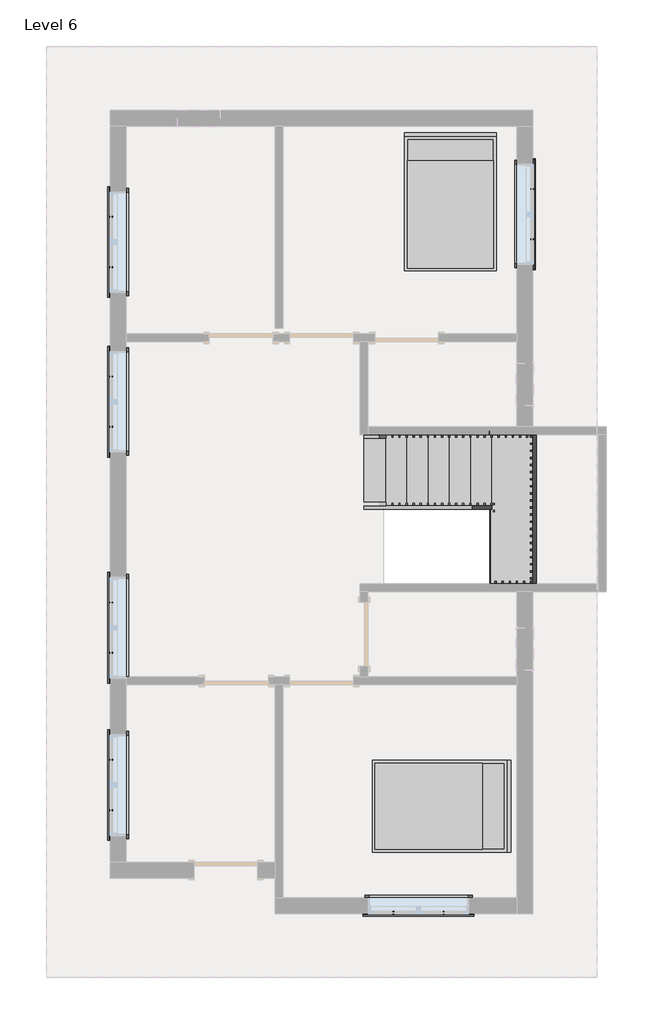
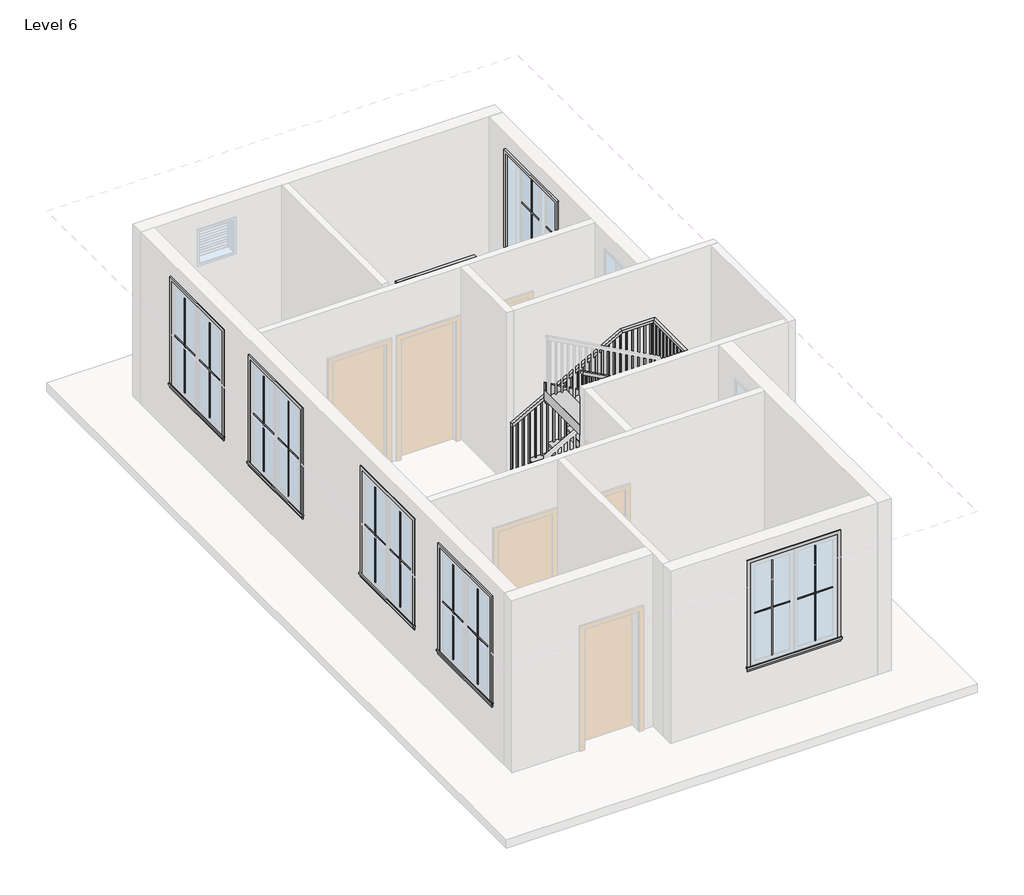
# One storey, part 2 of 2: 24 proxies, 5 members, 2 furniture elements, 1 railing, 1 stair flight.
"""IFC4 building model written with IfcOpenShell, lengths in millimetres."""

from ifc_helpers import new_model, si_unit, frame, origin, place, context, project, spatial, polyline, outline, extrude, faceted_brep, transform, mapped, element, save
from components import muntin_pattern_2x2_muntin_pattern_2x2_bff912c5, muntin_pattern_2x2_muntin_pattern_2x2_c2194282, trim_window_exterior_flat_with_sill_e04b3088, trim_window_interior_flat_picture_frame_2a7685fe, bed_17739_bed_17739_15c61121, stair_flight_57dbdc02

model = new_model("IFC4")

# Units and contexts
model_context = context("Model", 3, world=origin())
ifc_project = project(units=[si_unit("LENGTHUNIT", "METRE", prefix="MILLI")], contexts=[model_context])

# Site, building, storey
site = spatial("IfcSite", under=ifc_project)
building = spatial("IfcBuilding", under=site)
storey = spatial("IfcBuildingStorey", under=building, Name="Level 6", Elevation=12801.6)

# Proxies
placement = place(None, origin())
muntin_pattern_2x2_muntin_pattern_2x2_shape = muntin_pattern_2x2_muntin_pattern_2x2_bff912c5(model_context)
element("IfcBuildingElementProxy", 1, Name="Muntin Pattern_2x2 : Muntin Pattern_2x2", ObjectType="Muntin Pattern_2x2 : Muntin Pattern_2x2", at=placement, inside=storey, context=model_context, shape_type="MappedRepresentation", body=[
    mapped(muntin_pattern_2x2_muntin_pattern_2x2_shape, transform((-4796.6888307, -4528.6107799, 13785.85), x_axis=(0.0, 1.0, 0.0), y_axis=(-1.0, 0.0, 0.0), z_axis=(0.0, 0.0, 1.0))),
])
element("IfcBuildingElementProxy", 2, Name="Muntin Pattern_2x2 : Muntin Pattern_2x2", ObjectType="Muntin Pattern_2x2 : Muntin Pattern_2x2", at=placement, inside=storey, context=model_context, shape_type="MappedRepresentation", body=[
    mapped(muntin_pattern_2x2_muntin_pattern_2x2_shape, transform((-4796.6888307, -2274.3607799, 13785.85), x_axis=(0.0, 1.0, 0.0), y_axis=(-1.0, 0.0, 0.0), z_axis=(0.0, 0.0, 1.0))),
])
element("IfcBuildingElementProxy", 3, Name="Muntin Pattern_2x2 : Muntin Pattern_2x2", ObjectType="Muntin Pattern_2x2 : Muntin Pattern_2x2", at=placement, inside=storey, context=model_context, shape_type="MappedRepresentation", body=[
    mapped(muntin_pattern_2x2_muntin_pattern_2x2_shape, transform((-26.2513307, -6000.2232799, 13785.85), x_axis=(-1.0, 0.0, 0.0), y_axis=(0.0, -1.0, 0.0), z_axis=(0.0, 0.0, 1.0))),
])
element("IfcBuildingElementProxy", 4, Name="Muntin Pattern_2x2 : Muntin Pattern_2x2", ObjectType="Muntin Pattern_2x2 : Muntin Pattern_2x2", at=placement, inside=storey, context=model_context, shape_type="MappedRepresentation", body=[
    mapped(muntin_pattern_2x2_muntin_pattern_2x2_shape, transform((1242.1611693, 4370.9142201, 13785.85), x_axis=(0.0, -1.0, 0.0), y_axis=(1.0, 0.0, 0.0), z_axis=(0.0, 0.0, 1.0))),
])
element("IfcBuildingElementProxy", 5, Name="Muntin Pattern_2x2 : Muntin Pattern_2x2", ObjectType="Muntin Pattern_2x2 : Muntin Pattern_2x2", at=placement, inside=storey, context=model_context, shape_type="MappedRepresentation", body=[
    mapped(muntin_pattern_2x2_muntin_pattern_2x2_shape, transform((-4796.6888307, 3250.1392201, 13785.85), x_axis=(0.0, 1.0, 0.0), y_axis=(-1.0, 0.0, 0.0), z_axis=(0.0, 0.0, 1.0))),
])
element("IfcBuildingElementProxy", 6, Name="Muntin Pattern_2x2 : Muntin Pattern_2x2", ObjectType="Muntin Pattern_2x2 : Muntin Pattern_2x2", at=placement, inside=storey, context=model_context, shape_type="MappedRepresentation", body=[
    mapped(muntin_pattern_2x2_muntin_pattern_2x2_shape, transform((-4796.6888307, 964.1392201, 13785.85), x_axis=(0.0, 1.0, 0.0), y_axis=(-1.0, 0.0, 0.0), z_axis=(0.0, 0.0, 1.0))),
])
muntin_pattern_2x2_muntin_pattern_2x2_2_shape = muntin_pattern_2x2_muntin_pattern_2x2_c2194282(model_context)
element("IfcBuildingElementProxy", 7, Name="Muntin Pattern_2x2 : Muntin Pattern_2x2", ObjectType="Muntin Pattern_2x2 : Muntin Pattern_2x2", at=placement, inside=storey, context=model_context, shape_type="MappedRepresentation", body=[
    mapped(muntin_pattern_2x2_muntin_pattern_2x2_2_shape, transform((-4796.6888307, -3807.8857799, 13785.85), x_axis=(0.0, -1.0, 0.0), y_axis=(1.0, 0.0, 0.0), z_axis=(0.0, 0.0, 1.0))),
])
element("IfcBuildingElementProxy", 8, Name="Muntin Pattern_2x2 : Muntin Pattern_2x2", ObjectType="Muntin Pattern_2x2 : Muntin Pattern_2x2", at=placement, inside=storey, context=model_context, shape_type="MappedRepresentation", body=[
    mapped(muntin_pattern_2x2_muntin_pattern_2x2_2_shape, transform((-4796.6888307, -1553.6357799, 13785.85), x_axis=(0.0, -1.0, 0.0), y_axis=(1.0, 0.0, 0.0), z_axis=(0.0, 0.0, 1.0))),
])
element("IfcBuildingElementProxy", 9, Name="Muntin Pattern_2x2 : Muntin Pattern_2x2", ObjectType="Muntin Pattern_2x2 : Muntin Pattern_2x2", at=placement, inside=storey, context=model_context, shape_type="MappedRepresentation", body=[
    mapped(muntin_pattern_2x2_muntin_pattern_2x2_2_shape, transform((-746.9763307, -6000.2232799, 13785.85), x_axis=(1.0, 0.0, 0.0), y_axis=(0.0, 1.0, 0.0), z_axis=(0.0, 0.0, 1.0))),
])
element("IfcBuildingElementProxy", 10, Name="Muntin Pattern_2x2 : Muntin Pattern_2x2", ObjectType="Muntin Pattern_2x2 : Muntin Pattern_2x2", at=placement, inside=storey, context=model_context, shape_type="MappedRepresentation", body=[
    mapped(muntin_pattern_2x2_muntin_pattern_2x2_2_shape, transform((1242.1611693, 3650.1892201, 13785.85), x_axis=(0.0, 1.0, 0.0), y_axis=(-1.0, 0.0, 0.0), z_axis=(0.0, 0.0, 1.0))),
])
element("IfcBuildingElementProxy", 11, Name="Muntin Pattern_2x2 : Muntin Pattern_2x2", ObjectType="Muntin Pattern_2x2 : Muntin Pattern_2x2", at=placement, inside=storey, context=model_context, shape_type="MappedRepresentation", body=[
    mapped(muntin_pattern_2x2_muntin_pattern_2x2_2_shape, transform((-4796.6888307, 3970.8642201, 13785.85), x_axis=(0.0, -1.0, 0.0), y_axis=(1.0, 0.0, 0.0), z_axis=(0.0, 0.0, 1.0))),
])
element("IfcBuildingElementProxy", 12, Name="Muntin Pattern_2x2 : Muntin Pattern_2x2", ObjectType="Muntin Pattern_2x2 : Muntin Pattern_2x2", at=placement, inside=storey, context=model_context, shape_type="MappedRepresentation", body=[
    mapped(muntin_pattern_2x2_muntin_pattern_2x2_2_shape, transform((-4796.6888307, 1684.8642201, 13785.85), x_axis=(0.0, -1.0, 0.0), y_axis=(1.0, 0.0, 0.0), z_axis=(0.0, 0.0, 1.0))),
])
trim_window_exterior_flat_with_sill_shape = trim_window_exterior_flat_with_sill_e04b3088(model_context)
element("IfcBuildingElementProxy", 13, Name="Trim-Window-Exterior-Flat : with Sill", ObjectType="Trim-Window-Exterior-Flat : with Sill", at=placement, inside=storey, context=model_context, shape_type="MappedRepresentation", body=[
    mapped(trim_window_exterior_flat_with_sill_shape, transform((-4806.2138307, -4168.2482799, 15544.8), x_axis=(0.0, -1.0, 0.0), y_axis=(0.0, 0.0, 1.0), z_axis=(-1.0, 0.0, 0.0))),
])
element("IfcBuildingElementProxy", 14, Name="Trim-Window-Exterior-Flat : with Sill", ObjectType="Trim-Window-Exterior-Flat : with Sill", at=placement, inside=storey, context=model_context, shape_type="MappedRepresentation", body=[
    mapped(trim_window_exterior_flat_with_sill_shape, transform((-4806.2138307, -1913.9982799, 15544.8), x_axis=(0.0, -1.0, 0.0), y_axis=(0.0, 0.0, 1.0), z_axis=(-1.0, 0.0, 0.0))),
])
element("IfcBuildingElementProxy", 15, Name="Trim-Window-Exterior-Flat : with Sill", ObjectType="Trim-Window-Exterior-Flat : with Sill", at=placement, inside=storey, context=model_context, shape_type="MappedRepresentation", body=[
    mapped(trim_window_exterior_flat_with_sill_shape, transform((-386.6138307, -6009.7482799, 15544.8), x_axis=(1.0, 0.0, 0.0), y_axis=(0.0, 0.0, 1.0), z_axis=(0.0, -1.0, 0.0))),
])
element("IfcBuildingElementProxy", 16, Name="Trim-Window-Exterior-Flat : with Sill", ObjectType="Trim-Window-Exterior-Flat : with Sill", at=placement, inside=storey, context=model_context, shape_type="MappedRepresentation", body=[
    mapped(trim_window_exterior_flat_with_sill_shape, transform((1251.6861693, 4010.5517201, 15544.8), x_axis=(0.0, 1.0, 0.0), y_axis=(0.0, 0.0, 1.0), z_axis=(1.0, 0.0, 0.0))),
])
element("IfcBuildingElementProxy", 17, Name="Trim-Window-Exterior-Flat : with Sill", ObjectType="Trim-Window-Exterior-Flat : with Sill", at=placement, inside=storey, context=model_context, shape_type="MappedRepresentation", body=[
    mapped(trim_window_exterior_flat_with_sill_shape, transform((-4806.2138307, 3610.5017201, 15544.8), x_axis=(0.0, -1.0, 0.0), y_axis=(0.0, 0.0, 1.0), z_axis=(-1.0, 0.0, 0.0))),
])
element("IfcBuildingElementProxy", 18, Name="Trim-Window-Exterior-Flat : with Sill", ObjectType="Trim-Window-Exterior-Flat : with Sill", at=placement, inside=storey, context=model_context, shape_type="MappedRepresentation", body=[
    mapped(trim_window_exterior_flat_with_sill_shape, transform((-4806.2138307, 1324.5017201, 15544.8), x_axis=(0.0, -1.0, 0.0), y_axis=(0.0, 0.0, 1.0), z_axis=(-1.0, 0.0, 0.0))),
])
trim_window_interior_flat_picture_frame_shape = trim_window_interior_flat_picture_frame_2a7685fe(model_context)
element("IfcBuildingElementProxy", 19, Name="Trim-Window-Interior-Flat : Picture Frame", ObjectType="Trim-Window-Interior-Flat : Picture Frame", at=placement, inside=storey, context=model_context, shape_type="MappedRepresentation", body=[
    mapped(trim_window_interior_flat_picture_frame_shape, transform((-4577.6138307, -4168.2482799, 15544.8), x_axis=(0.0, 1.0, 0.0), y_axis=(0.0, 0.0, 1.0), z_axis=(1.0, 0.0, 0.0))),
])
element("IfcBuildingElementProxy", 20, Name="Trim-Window-Interior-Flat : Picture Frame", ObjectType="Trim-Window-Interior-Flat : Picture Frame", at=placement, inside=storey, context=model_context, shape_type="MappedRepresentation", body=[
    mapped(trim_window_interior_flat_picture_frame_shape, transform((-4577.6138307, -1913.9982799, 15544.8), x_axis=(0.0, 1.0, 0.0), y_axis=(0.0, 0.0, 1.0), z_axis=(1.0, 0.0, 0.0))),
])
element("IfcBuildingElementProxy", 21, Name="Trim-Window-Interior-Flat : Picture Frame", ObjectType="Trim-Window-Interior-Flat : Picture Frame", at=placement, inside=storey, context=model_context, shape_type="MappedRepresentation", body=[
    mapped(trim_window_interior_flat_picture_frame_shape, transform((-386.6138307, -5781.1482799, 15544.8), x_axis=(-1.0, 0.0, 0.0), y_axis=(0.0, 0.0, 1.0), z_axis=(0.0, 1.0, 0.0))),
])
element("IfcBuildingElementProxy", 22, Name="Trim-Window-Interior-Flat : Picture Frame", ObjectType="Trim-Window-Interior-Flat : Picture Frame", at=placement, inside=storey, context=model_context, shape_type="MappedRepresentation", body=[
    mapped(trim_window_interior_flat_picture_frame_shape, transform((1023.0861693, 4010.5517201, 15544.8), x_axis=(0.0, -1.0, 0.0), y_axis=(0.0, 0.0, 1.0), z_axis=(-1.0, 0.0, 0.0))),
])
element("IfcBuildingElementProxy", 23, Name="Trim-Window-Interior-Flat : Picture Frame", ObjectType="Trim-Window-Interior-Flat : Picture Frame", at=placement, inside=storey, context=model_context, shape_type="MappedRepresentation", body=[
    mapped(trim_window_interior_flat_picture_frame_shape, transform((-4577.6138307, 3610.5017201, 15544.8), x_axis=(0.0, 1.0, 0.0), y_axis=(0.0, 0.0, 1.0), z_axis=(1.0, 0.0, 0.0))),
])
element("IfcBuildingElementProxy", 24, Name="Trim-Window-Interior-Flat : Picture Frame", ObjectType="Trim-Window-Interior-Flat : Picture Frame", at=placement, inside=storey, context=model_context, shape_type="MappedRepresentation", body=[
    mapped(trim_window_interior_flat_picture_frame_shape, transform((-4577.6138307, 1324.5017201, 15544.8), x_axis=(0.0, 1.0, 0.0), y_axis=(0.0, 0.0, 1.0), z_axis=(1.0, 0.0, 0.0))),
])

# Furniture
bed_17739_bed_17739_shape = bed_17739_bed_17739_15c61121(model_context)
element("IfcFurniture", 25, ObjectType="Bed_17739 : Bed_17739", at=placement, inside=storey, context=model_context, shape_type="MappedRepresentation", body=[
    mapped(bed_17739_bed_17739_shape, transform((70.5861693, 4162.9517201, 12801.6), x_axis=(1.0, 0.0, 0.0), y_axis=(0.0, 1.0, 0.0), z_axis=(0.0, 0.0, 1.0))),
])
element("IfcFurniture", 26, ObjectType="Bed_17739 : Bed_17739", at=placement, inside=storey, context=model_context, shape_type="MappedRepresentation", body=[
    mapped(bed_17739_bed_17739_shape, transform((-81.8138307, -4473.0482799, 12801.6), x_axis=(0.0, -1.0, 0.0), y_axis=(1.0, 0.0, 0.0), z_axis=(0.0, 0.0, 1.0))),
])

# Members
element("IfcMember", 27, ObjectType="Stringer - 2\" Width", at=placement, inside=storey, context=model_context, shape_type="SweptSolid", body=[
    extrude(outline(polyline([(13005.670617, -1167.6638307), (12801.6, -1167.6638307), (12801.6, -907.3693279), (14001.0752762, 1251.6861693), (14063.1333333, 1251.6861693), (14063.1333333, 735.7690587), (13005.670617, -1167.6638307)])), frame((0.0, 848.2517201, 0.0), z_axis=(0.0, 1.0, 0.0), x_axis=(0.0, 0.0, 1.0)), (0.0, 0.0, 1.0), 50.8),
])
element("IfcMember", 28, ObjectType="Stringer - 2\" Width", at=placement, inside=storey, context=model_context, shape_type="SweptSolid", body=[
    extrude(outline(polyline([(1251.6861693, 899.0517201), (1302.4861693, 899.0517201), (1302.4861693, -1285.3482799), (1251.6861693, -1285.3482799), (1251.6861693, 899.0517201)])), frame((0.0, 0.0, 13758.3333333), z_axis=(0.0, 0.0, 1.0), x_axis=(1.0, 0.0, 0.0)), (0.0, 0.0, 1.0), 304.8),
])
element("IfcMember", 29, ObjectType="Stringer - 2\" Width", at=placement, inside=storey, context=model_context, shape_type="SweptSolid", body=[
    extrude(outline(polyline([(13758.3333333, 1302.4861693), (13841.7539503, 1302.4861693), (15224.6428392, -1186.7138307), (14875.9641651, -1186.7138307), (13758.3333333, 825.0216665), (13758.3333333, 1302.4861693)])), frame((0.0, -1336.1482799, 0.0), z_axis=(0.0, 1.0, 0.0), x_axis=(0.0, 0.0, 1.0)), (0.0, 0.0, 1.0), 50.8),
])
element("IfcMember", 30, ObjectType="Stringer - 2\" Width", at=placement, inside=storey, context=model_context, shape_type="SweptSolid", body=[
    extrude(outline(polyline([(13005.670617, -1167.6638307), (12801.6, -1167.6638307), (12801.6, -907.3693279), (13648.2974984, 616.6861693), (13996.9761726, 616.6861693), (13005.670617, -1167.6638307)])), frame((0.0, -218.5482799, 0.0), z_axis=(0.0, 1.0, 0.0), x_axis=(0.0, 0.0, 1.0)), (0.0, 0.0, 1.0), 50.8),
])
element("IfcMember", 31, ObjectType="Stringer - 2\" Width", at=placement, inside=storey, context=model_context, shape_type="SweptSolid", body=[
    extrude(outline(polyline([(13845.853054, 667.4861693), (14194.5317281, 667.4861693), (15224.6428392, -1186.7138307), (14875.9641651, -1186.7138307), (13845.853054, 667.4861693)])), frame((0.0, -218.5482799, 0.0), z_axis=(0.0, 1.0, 0.0), x_axis=(0.0, 0.0, 1.0)), (0.0, 0.0, 1.0), 50.8),
])

# Railing
element("IfcRailing", 32, ObjectType="Handrail - Rectangular", at=placement, inside=storey, context=model_context, shape_type="SolidModel", body=[
    faceted_brep([(-1167.6638307, 848.2517201, 13885.3333333), (-1167.6638307, 848.2517201, 13827.2675836), (-1167.6638307, 797.4517201, 13827.2675836), (-1167.6638307, 797.4517201, 13885.3333333), (667.4861693, 848.2517201, 14901.3333333), (680.6099298, 848.2517201, 14850.5333333), (680.6099298, 797.4517201, 14850.5333333), (667.4861693, 797.4517201, 14901.3333333), (1251.6861693, 848.2517201, 14901.3333333), (1251.6861693, 848.2517201, 14850.5333333), (1200.8861693, 797.4517201, 14850.5333333), (1200.8861693, 797.4517201, 14901.3333333), (1251.6861693, -1285.3482799, 14901.3333333), (1251.6861693, -1285.3482799, 14850.5333333), (1200.8861693, -1234.5482799, 14850.5333333), (1200.8861693, -1234.5482799, 14901.3333333), (976.5195026, -1285.3482799, 14901.3333333), (963.5139215, -1285.3482799, 14850.5333333), (963.5139215, -1234.5482799, 14850.5333333), (976.5195026, -1234.5482799, 14901.3333333), (-1186.7138307, -1285.3482799, 16086.6666667), (-1186.7138307, -1234.5482799, 16086.6666667), (-1186.7138307, -1234.5482799, 16028.7403208), (-1186.7138307, -1285.3482799, 16028.7403208)], [[[0, 1, 2, 3]], [[1, 0, 4, 5]], [[2, 1, 5, 6]], [[3, 2, 6, 7]], [[0, 3, 7, 4]], [[5, 4, 8, 9]], [[6, 5, 9, 10]], [[7, 6, 10, 11]], [[4, 7, 11, 8]], [[9, 8, 12, 13]], [[10, 9, 13, 14]], [[11, 10, 14, 15]], [[8, 11, 15, 12]], [[13, 12, 16, 17]], [[14, 13, 17, 18]], [[15, 14, 18, 19]], [[12, 15, 19, 16]], [[20, 21, 22, 23]], [[17, 16, 20, 23]], [[18, 17, 23, 22]], [[19, 18, 22, 21]], [[16, 19, 21, 20]]]),
    extrude(outline(polyline([(15992.2060742, -1120.0388307), (15002.9333333, -1120.0388307), (15002.9333333, -1100.9888307), (15981.7677181, -1100.9888307), (15992.2060742, -1120.0388307)])), frame((0.0, -1269.4732799, 0.0), z_axis=(0.0, 1.0, 0.0), x_axis=(0.0, 0.0, 1.0)), (0.0, 0.0, 1.0), 19.05),
    extrude(outline(polyline([(15936.5348414, -1018.4388307), (15002.9333333, -1018.4388307), (15002.9333333, -999.3888307), (15926.0964852, -999.3888307), (15936.5348414, -1018.4388307)])), frame((0.0, -1269.4732799, 0.0), z_axis=(0.0, 1.0, 0.0), x_axis=(0.0, 0.0, 1.0)), (0.0, 0.0, 1.0), 19.05),
    extrude(outline(polyline([(15880.8636085, -916.8388307), (15002.9333333, -916.8388307), (15002.9333333, -897.7888307), (15870.4252523, -897.7888307), (15880.8636085, -916.8388307)])), frame((0.0, -1269.4732799, 0.0), z_axis=(0.0, 1.0, 0.0), x_axis=(0.0, 0.0, 1.0)), (0.0, 0.0, 1.0), 19.05),
    extrude(outline(polyline([(15825.1923756, -815.2388307), (14833.6, -815.2388307), (14833.6, -796.1888307), (15814.7540195, -796.1888307), (15825.1923756, -815.2388307)])), frame((0.0, -1269.4732799, 0.0), z_axis=(0.0, 1.0, 0.0), x_axis=(0.0, 0.0, 1.0)), (0.0, 0.0, 1.0), 19.05),
    extrude(outline(polyline([(15769.5211427, -713.6388307), (14833.6, -713.6388307), (14833.6, -694.5888307), (15759.0827866, -694.5888307), (15769.5211427, -713.6388307)])), frame((0.0, -1269.4732799, 0.0), z_axis=(0.0, 1.0, 0.0), x_axis=(0.0, 0.0, 1.0)), (0.0, 0.0, 1.0), 19.05),
    extrude(outline(polyline([(15713.8499099, -612.0388307), (14833.6, -612.0388307), (14833.6, -592.9888307), (15703.4115537, -592.9888307), (15713.8499099, -612.0388307)])), frame((0.0, -1269.4732799, 0.0), z_axis=(0.0, 1.0, 0.0), x_axis=(0.0, 0.0, 1.0)), (0.0, 0.0, 1.0), 19.05),
    extrude(outline(polyline([(15658.178677, -510.4388307), (14664.2666667, -510.4388307), (14664.2666667, -491.3888307), (15647.7403208, -491.3888307), (15658.178677, -510.4388307)])), frame((0.0, -1269.4732799, 0.0), z_axis=(0.0, 1.0, 0.0), x_axis=(0.0, 0.0, 1.0)), (0.0, 0.0, 1.0), 19.05),
    extrude(outline(polyline([(15602.5074441, -408.8388307), (14664.2666667, -408.8388307), (14664.2666667, -389.7888307), (15592.0690879, -389.7888307), (15602.5074441, -408.8388307)])), frame((0.0, -1269.4732799, 0.0), z_axis=(0.0, 1.0, 0.0), x_axis=(0.0, 0.0, 1.0)), (0.0, 0.0, 1.0), 19.05),
    extrude(outline(polyline([(15546.8362112, -307.2388307), (14664.2666667, -307.2388307), (14664.2666667, -288.1888307), (15536.3978551, -288.1888307), (15546.8362112, -307.2388307)])), frame((0.0, -1269.4732799, 0.0), z_axis=(0.0, 1.0, 0.0), x_axis=(0.0, 0.0, 1.0)), (0.0, 0.0, 1.0), 19.05),
    extrude(outline(polyline([(15491.1649784, -205.6388307), (14494.9333333, -205.6388307), (14494.9333333, -186.5888307), (15480.7266222, -186.5888307), (15491.1649784, -205.6388307)])), frame((0.0, -1269.4732799, 0.0), z_axis=(0.0, 1.0, 0.0), x_axis=(0.0, 0.0, 1.0)), (0.0, 0.0, 1.0), 19.05),
    extrude(outline(polyline([(15435.4937455, -104.0388307), (14494.9333333, -104.0388307), (14494.9333333, -84.9888307), (15425.0553893, -84.9888307), (15435.4937455, -104.0388307)])), frame((0.0, -1269.4732799, 0.0), z_axis=(0.0, 1.0, 0.0), x_axis=(0.0, 0.0, 1.0)), (0.0, 0.0, 1.0), 19.05),
    extrude(outline(polyline([(15379.8225126, -2.4388307), (14494.9333333, -2.4388307), (14494.9333333, 16.6111693), (15369.3841564, 16.6111693), (15379.8225126, -2.4388307)])), frame((0.0, -1269.4732799, 0.0), z_axis=(0.0, 1.0, 0.0), x_axis=(0.0, 0.0, 1.0)), (0.0, 0.0, 1.0), 19.05),
    extrude(outline(polyline([(15324.1512797, 99.1611693), (14325.6, 99.1611693), (14325.6, 118.2111693), (15313.7129236, 118.2111693), (15324.1512797, 99.1611693)])), frame((0.0, -1269.4732799, 0.0), z_axis=(0.0, 1.0, 0.0), x_axis=(0.0, 0.0, 1.0)), (0.0, 0.0, 1.0), 19.05),
    extrude(outline(polyline([(15268.4800469, 200.7611693), (14325.6, 200.7611693), (14325.6, 219.8111693), (15258.0416907, 219.8111693), (15268.4800469, 200.7611693)])), frame((0.0, -1269.4732799, 0.0), z_axis=(0.0, 1.0, 0.0), x_axis=(0.0, 0.0, 1.0)), (0.0, 0.0, 1.0), 19.05),
    extrude(outline(polyline([(15212.808814, 302.3611693), (14325.6, 302.3611693), (14325.6, 321.4111693), (15202.3704578, 321.4111693), (15212.808814, 302.3611693)])), frame((0.0, -1269.4732799, 0.0), z_axis=(0.0, 1.0, 0.0), x_axis=(0.0, 0.0, 1.0)), (0.0, 0.0, 1.0), 19.05),
    extrude(outline(polyline([(15157.1375811, 403.9611693), (14156.2666667, 403.9611693), (14156.2666667, 423.0111693), (15146.6992249, 423.0111693), (15157.1375811, 403.9611693)])), frame((0.0, -1269.4732799, 0.0), z_axis=(0.0, 1.0, 0.0), x_axis=(0.0, 0.0, 1.0)), (0.0, 0.0, 1.0), 19.05),
    extrude(outline(polyline([(15101.4663482, 505.5611693), (14156.2666667, 505.5611693), (14156.2666667, 524.6111693), (15091.0279921, 524.6111693), (15101.4663482, 505.5611693)])), frame((0.0, -1269.4732799, 0.0), z_axis=(0.0, 1.0, 0.0), x_axis=(0.0, 0.0, 1.0)), (0.0, 0.0, 1.0), 19.05),
    extrude(outline(polyline([(15045.7951153, 607.1611693), (14156.2666667, 607.1611693), (14156.2666667, 626.2111693), (15035.3567592, 626.2111693), (15045.7951153, 607.1611693)])), frame((0.0, -1269.4732799, 0.0), z_axis=(0.0, 1.0, 0.0), x_axis=(0.0, 0.0, 1.0)), (0.0, 0.0, 1.0), 19.05),
    extrude(outline(polyline([(14990.1238825, 708.7611693), (13986.9333333, 708.7611693), (13986.9333333, 727.8111693), (14979.6855263, 727.8111693), (14990.1238825, 708.7611693)])), frame((0.0, -1269.4732799, 0.0), z_axis=(0.0, 1.0, 0.0), x_axis=(0.0, 0.0, 1.0)), (0.0, 0.0, 1.0), 19.05),
    extrude(outline(polyline([(14934.4526496, 810.3611693), (13986.9333333, 810.3611693), (13986.9333333, 829.4111693), (14924.0142934, 829.4111693), (14934.4526496, 810.3611693)])), frame((0.0, -1269.4732799, 0.0), z_axis=(0.0, 1.0, 0.0), x_axis=(0.0, 0.0, 1.0)), (0.0, 0.0, 1.0), 19.05),
    extrude(outline(polyline([(14878.7814167, 911.9611693), (13986.9333333, 911.9611693), (13986.9333333, 931.0111693), (14868.3430606, 931.0111693), (14878.7814167, 911.9611693)])), frame((0.0, -1269.4732799, 0.0), z_axis=(0.0, 1.0, 0.0), x_axis=(0.0, 0.0, 1.0)), (0.0, 0.0, 1.0), 19.05),
    extrude(outline(polyline([(1032.6111693, -1269.4732799), (1013.5611693, -1269.4732799), (1013.5611693, -1250.4232799), (1032.6111693, -1250.4232799), (1032.6111693, -1269.4732799)])), frame((0.0, 0.0, 13986.9333333), z_axis=(0.0, 0.0, 1.0), x_axis=(1.0, 0.0, 0.0)), (0.0, 0.0, 1.0), 863.6),
    extrude(outline(polyline([(1134.2111693, -1269.4732799), (1115.1611693, -1269.4732799), (1115.1611693, -1250.4232799), (1134.2111693, -1250.4232799), (1134.2111693, -1269.4732799)])), frame((0.0, 0.0, 13986.9333333), z_axis=(0.0, 0.0, 1.0), x_axis=(1.0, 0.0, 0.0)), (0.0, 0.0, 1.0), 863.6),
    extrude(outline(polyline([(1235.8111693, -1199.6232799), (1235.8111693, -1218.6732799), (1216.7611693, -1218.6732799), (1216.7611693, -1199.6232799), (1235.8111693, -1199.6232799)])), frame((0.0, 0.0, 13986.9333333), z_axis=(0.0, 0.0, 1.0), x_axis=(1.0, 0.0, 0.0)), (0.0, 0.0, 1.0), 863.6),
    extrude(outline(polyline([(1235.8111693, -1098.0232799), (1235.8111693, -1117.0732799), (1216.7611693, -1117.0732799), (1216.7611693, -1098.0232799), (1235.8111693, -1098.0232799)])), frame((0.0, 0.0, 13986.9333333), z_axis=(0.0, 0.0, 1.0), x_axis=(1.0, 0.0, 0.0)), (0.0, 0.0, 1.0), 863.6),
    extrude(outline(polyline([(1235.8111693, -996.4232799), (1235.8111693, -1015.4732799), (1216.7611693, -1015.4732799), (1216.7611693, -996.4232799), (1235.8111693, -996.4232799)])), frame((0.0, 0.0, 13986.9333333), z_axis=(0.0, 0.0, 1.0), x_axis=(1.0, 0.0, 0.0)), (0.0, 0.0, 1.0), 863.6),
    extrude(outline(polyline([(1235.8111693, -894.8232799), (1235.8111693, -913.8732799), (1216.7611693, -913.8732799), (1216.7611693, -894.8232799), (1235.8111693, -894.8232799)])), frame((0.0, 0.0, 13986.9333333), z_axis=(0.0, 0.0, 1.0), x_axis=(1.0, 0.0, 0.0)), (0.0, 0.0, 1.0), 863.6),
    extrude(outline(polyline([(1235.8111693, -793.2232799), (1235.8111693, -812.2732799), (1216.7611693, -812.2732799), (1216.7611693, -793.2232799), (1235.8111693, -793.2232799)])), frame((0.0, 0.0, 13986.9333333), z_axis=(0.0, 0.0, 1.0), x_axis=(1.0, 0.0, 0.0)), (0.0, 0.0, 1.0), 863.6),
    extrude(outline(polyline([(1235.8111693, -691.6232799), (1235.8111693, -710.6732799), (1216.7611693, -710.6732799), (1216.7611693, -691.6232799), (1235.8111693, -691.6232799)])), frame((0.0, 0.0, 13986.9333333), z_axis=(0.0, 0.0, 1.0), x_axis=(1.0, 0.0, 0.0)), (0.0, 0.0, 1.0), 863.6),
    extrude(outline(polyline([(1235.8111693, -590.0232799), (1235.8111693, -609.0732799), (1216.7611693, -609.0732799), (1216.7611693, -590.0232799), (1235.8111693, -590.0232799)])), frame((0.0, 0.0, 13986.9333333), z_axis=(0.0, 0.0, 1.0), x_axis=(1.0, 0.0, 0.0)), (0.0, 0.0, 1.0), 863.6),
    extrude(outline(polyline([(1235.8111693, -488.4232799), (1235.8111693, -507.4732799), (1216.7611693, -507.4732799), (1216.7611693, -488.4232799), (1235.8111693, -488.4232799)])), frame((0.0, 0.0, 13986.9333333), z_axis=(0.0, 0.0, 1.0), x_axis=(1.0, 0.0, 0.0)), (0.0, 0.0, 1.0), 863.6),
    extrude(outline(polyline([(1235.8111693, -386.8232799), (1235.8111693, -405.8732799), (1216.7611693, -405.8732799), (1216.7611693, -386.8232799), (1235.8111693, -386.8232799)])), frame((0.0, 0.0, 13986.9333333), z_axis=(0.0, 0.0, 1.0), x_axis=(1.0, 0.0, 0.0)), (0.0, 0.0, 1.0), 863.6),
    extrude(outline(polyline([(1235.8111693, -285.2232799), (1235.8111693, -304.2732799), (1216.7611693, -304.2732799), (1216.7611693, -285.2232799), (1235.8111693, -285.2232799)])), frame((0.0, 0.0, 13986.9333333), z_axis=(0.0, 0.0, 1.0), x_axis=(1.0, 0.0, 0.0)), (0.0, 0.0, 1.0), 863.6),
    extrude(outline(polyline([(1235.8111693, -183.6232799), (1235.8111693, -202.6732799), (1216.7611693, -202.6732799), (1216.7611693, -183.6232799), (1235.8111693, -183.6232799)])), frame((0.0, 0.0, 13986.9333333), z_axis=(0.0, 0.0, 1.0), x_axis=(1.0, 0.0, 0.0)), (0.0, 0.0, 1.0), 863.6),
    extrude(outline(polyline([(1235.8111693, -82.0232799), (1235.8111693, -101.0732799), (1216.7611693, -101.0732799), (1216.7611693, -82.0232799), (1235.8111693, -82.0232799)])), frame((0.0, 0.0, 13986.9333333), z_axis=(0.0, 0.0, 1.0), x_axis=(1.0, 0.0, 0.0)), (0.0, 0.0, 1.0), 863.6),
    extrude(outline(polyline([(1235.8111693, 19.5767201), (1235.8111693, 0.5267201), (1216.7611693, 0.5267201), (1216.7611693, 19.5767201), (1235.8111693, 19.5767201)])), frame((0.0, 0.0, 13986.9333333), z_axis=(0.0, 0.0, 1.0), x_axis=(1.0, 0.0, 0.0)), (0.0, 0.0, 1.0), 863.6),
    extrude(outline(polyline([(1235.8111693, 121.1767201), (1235.8111693, 102.1267201), (1216.7611693, 102.1267201), (1216.7611693, 121.1767201), (1235.8111693, 121.1767201)])), frame((0.0, 0.0, 13986.9333333), z_axis=(0.0, 0.0, 1.0), x_axis=(1.0, 0.0, 0.0)), (0.0, 0.0, 1.0), 863.6),
    extrude(outline(polyline([(1235.8111693, 222.7767201), (1235.8111693, 203.7267201), (1216.7611693, 203.7267201), (1216.7611693, 222.7767201), (1235.8111693, 222.7767201)])), frame((0.0, 0.0, 13986.9333333), z_axis=(0.0, 0.0, 1.0), x_axis=(1.0, 0.0, 0.0)), (0.0, 0.0, 1.0), 863.6),
    extrude(outline(polyline([(1235.8111693, 324.3767201), (1235.8111693, 305.3267201), (1216.7611693, 305.3267201), (1216.7611693, 324.3767201), (1235.8111693, 324.3767201)])), frame((0.0, 0.0, 13986.9333333), z_axis=(0.0, 0.0, 1.0), x_axis=(1.0, 0.0, 0.0)), (0.0, 0.0, 1.0), 863.6),
    extrude(outline(polyline([(1235.8111693, 425.9767201), (1235.8111693, 406.9267201), (1216.7611693, 406.9267201), (1216.7611693, 425.9767201), (1235.8111693, 425.9767201)])), frame((0.0, 0.0, 13986.9333333), z_axis=(0.0, 0.0, 1.0), x_axis=(1.0, 0.0, 0.0)), (0.0, 0.0, 1.0), 863.6),
    extrude(outline(polyline([(1235.8111693, 527.5767201), (1235.8111693, 508.5267201), (1216.7611693, 508.5267201), (1216.7611693, 527.5767201), (1235.8111693, 527.5767201)])), frame((0.0, 0.0, 13986.9333333), z_axis=(0.0, 0.0, 1.0), x_axis=(1.0, 0.0, 0.0)), (0.0, 0.0, 1.0), 863.6),
    extrude(outline(polyline([(1235.8111693, 629.1767201), (1235.8111693, 610.1267201), (1216.7611693, 610.1267201), (1216.7611693, 629.1767201), (1235.8111693, 629.1767201)])), frame((0.0, 0.0, 13986.9333333), z_axis=(0.0, 0.0, 1.0), x_axis=(1.0, 0.0, 0.0)), (0.0, 0.0, 1.0), 863.6),
    extrude(outline(polyline([(1235.8111693, 730.7767201), (1235.8111693, 711.7267201), (1216.7611693, 711.7267201), (1216.7611693, 730.7767201), (1235.8111693, 730.7767201)])), frame((0.0, 0.0, 13986.9333333), z_axis=(0.0, 0.0, 1.0), x_axis=(1.0, 0.0, 0.0)), (0.0, 0.0, 1.0), 863.6),
    extrude(outline(polyline([(1159.6111693, 832.3767201), (1178.6611693, 832.3767201), (1178.6611693, 813.3267201), (1159.6111693, 813.3267201), (1159.6111693, 832.3767201)])), frame((0.0, 0.0, 13986.9333333), z_axis=(0.0, 0.0, 1.0), x_axis=(1.0, 0.0, 0.0)), (0.0, 0.0, 1.0), 863.6),
    extrude(outline(polyline([(1058.0111693, 832.3767201), (1077.0611693, 832.3767201), (1077.0611693, 813.3267201), (1058.0111693, 813.3267201), (1058.0111693, 832.3767201)])), frame((0.0, 0.0, 13986.9333333), z_axis=(0.0, 0.0, 1.0), x_axis=(1.0, 0.0, 0.0)), (0.0, 0.0, 1.0), 863.6),
    extrude(outline(polyline([(956.4111693, 832.3767201), (975.4611693, 832.3767201), (975.4611693, 813.3267201), (956.4111693, 813.3267201), (956.4111693, 832.3767201)])), frame((0.0, 0.0, 13986.9333333), z_axis=(0.0, 0.0, 1.0), x_axis=(1.0, 0.0, 0.0)), (0.0, 0.0, 1.0), 863.6),
    extrude(outline(polyline([(854.8111693, 832.3767201), (873.8611693, 832.3767201), (873.8611693, 813.3267201), (854.8111693, 813.3267201), (854.8111693, 832.3767201)])), frame((0.0, 0.0, 13986.9333333), z_axis=(0.0, 0.0, 1.0), x_axis=(1.0, 0.0, 0.0)), (0.0, 0.0, 1.0), 863.6),
    extrude(outline(polyline([(753.2111693, 832.3767201), (772.2611693, 832.3767201), (772.2611693, 813.3267201), (753.2111693, 813.3267201), (753.2111693, 832.3767201)])), frame((0.0, 0.0, 13986.9333333), z_axis=(0.0, 0.0, 1.0), x_axis=(1.0, 0.0, 0.0)), (0.0, 0.0, 1.0), 863.6),
    extrude(outline(polyline([(14834.4786562, 651.6111693), (13817.6, 651.6111693), (13817.6, 670.6611693), (14845.025369, 670.6611693), (14834.4786562, 651.6111693)])), frame((0.0, 813.3267201, 0.0), z_axis=(0.0, 1.0, 0.0), x_axis=(0.0, 0.0, 1.0)), (0.0, 0.0, 1.0), 19.05),
    extrude(outline(polyline([(14778.2295213, 550.0111693), (13817.6, 550.0111693), (13817.6, 569.0611693), (14788.7762341, 569.0611693), (14778.2295213, 550.0111693)])), frame((0.0, 813.3267201, 0.0), z_axis=(0.0, 1.0, 0.0), x_axis=(0.0, 0.0, 1.0)), (0.0, 0.0, 1.0), 19.05),
    extrude(outline(polyline([(14721.9803863, 448.4111693), (13817.6, 448.4111693), (13817.6, 467.4611693), (14732.5270991, 467.4611693), (14721.9803863, 448.4111693)])), frame((0.0, 813.3267201, 0.0), z_axis=(0.0, 1.0, 0.0), x_axis=(0.0, 0.0, 1.0)), (0.0, 0.0, 1.0), 19.05),
    extrude(outline(polyline([(14665.7312514, 346.8111693), (13648.2666667, 346.8111693), (13648.2666667, 365.8611693), (14676.2779642, 365.8611693), (14665.7312514, 346.8111693)])), frame((0.0, 813.3267201, 0.0), z_axis=(0.0, 1.0, 0.0), x_axis=(0.0, 0.0, 1.0)), (0.0, 0.0, 1.0), 19.05),
    extrude(outline(polyline([(14609.4821164, 245.2111693), (13648.2666667, 245.2111693), (13648.2666667, 264.2611693), (14620.0288292, 264.2611693), (14609.4821164, 245.2111693)])), frame((0.0, 813.3267201, 0.0), z_axis=(0.0, 1.0, 0.0), x_axis=(0.0, 0.0, 1.0)), (0.0, 0.0, 1.0), 19.05),
    extrude(outline(polyline([(14553.2329815, 143.6111693), (13648.2666667, 143.6111693), (13648.2666667, 162.6611693), (14563.7796943, 162.6611693), (14553.2329815, 143.6111693)])), frame((0.0, 813.3267201, 0.0), z_axis=(0.0, 1.0, 0.0), x_axis=(0.0, 0.0, 1.0)), (0.0, 0.0, 1.0), 19.05),
    extrude(outline(polyline([(14496.9838465, 42.0111693), (13478.9333333, 42.0111693), (13478.9333333, 61.0611693), (14507.5305593, 61.0611693), (14496.9838465, 42.0111693)])), frame((0.0, 813.3267201, 0.0), z_axis=(0.0, 1.0, 0.0), x_axis=(0.0, 0.0, 1.0)), (0.0, 0.0, 1.0), 19.05),
    extrude(outline(polyline([(14440.7347116, -59.5888307), (13478.9333333, -59.5888307), (13478.9333333, -40.5388307), (14451.2814244, -40.5388307), (14440.7347116, -59.5888307)])), frame((0.0, 813.3267201, 0.0), z_axis=(0.0, 1.0, 0.0), x_axis=(0.0, 0.0, 1.0)), (0.0, 0.0, 1.0), 19.05),
    extrude(outline(polyline([(14384.4855766, -161.1888307), (13478.9333333, -161.1888307), (13478.9333333, -142.1388307), (14395.0322895, -142.1388307), (14384.4855766, -161.1888307)])), frame((0.0, 813.3267201, 0.0), z_axis=(0.0, 1.0, 0.0), x_axis=(0.0, 0.0, 1.0)), (0.0, 0.0, 1.0), 19.05),
    extrude(outline(polyline([(14328.2364417, -262.7888307), (13309.6, -262.7888307), (13309.6, -243.7388307), (14338.7831545, -243.7388307), (14328.2364417, -262.7888307)])), frame((0.0, 813.3267201, 0.0), z_axis=(0.0, 1.0, 0.0), x_axis=(0.0, 0.0, 1.0)), (0.0, 0.0, 1.0), 19.05),
    extrude(outline(polyline([(14271.9873068, -364.3888307), (13309.6, -364.3888307), (13309.6, -345.3388307), (14282.5340196, -345.3388307), (14271.9873068, -364.3888307)])), frame((0.0, 813.3267201, 0.0), z_axis=(0.0, 1.0, 0.0), x_axis=(0.0, 0.0, 1.0)), (0.0, 0.0, 1.0), 19.05),
    extrude(outline(polyline([(14215.7381718, -465.9888307), (13309.6, -465.9888307), (13309.6, -446.9388307), (14226.2848846, -446.9388307), (14215.7381718, -465.9888307)])), frame((0.0, 813.3267201, 0.0), z_axis=(0.0, 1.0, 0.0), x_axis=(0.0, 0.0, 1.0)), (0.0, 0.0, 1.0), 19.05),
    extrude(outline(polyline([(14159.4890369, -567.5888307), (13140.2666667, -567.5888307), (13140.2666667, -548.5388307), (14170.0357497, -548.5388307), (14159.4890369, -567.5888307)])), frame((0.0, 813.3267201, 0.0), z_axis=(0.0, 1.0, 0.0), x_axis=(0.0, 0.0, 1.0)), (0.0, 0.0, 1.0), 19.05),
    extrude(outline(polyline([(14103.2399019, -669.1888307), (13140.2666667, -669.1888307), (13140.2666667, -650.1388307), (14113.7866147, -650.1388307), (14103.2399019, -669.1888307)])), frame((0.0, 813.3267201, 0.0), z_axis=(0.0, 1.0, 0.0), x_axis=(0.0, 0.0, 1.0)), (0.0, 0.0, 1.0), 19.05),
    extrude(outline(polyline([(14046.990767, -770.7888307), (13140.2666667, -770.7888307), (13140.2666667, -751.7388307), (14057.5374798, -751.7388307), (14046.990767, -770.7888307)])), frame((0.0, 813.3267201, 0.0), z_axis=(0.0, 1.0, 0.0), x_axis=(0.0, 0.0, 1.0)), (0.0, 0.0, 1.0), 19.05),
    extrude(outline(polyline([(13990.741632, -872.3888307), (12970.9333333, -872.3888307), (12970.9333333, -853.3388307), (14001.2883448, -853.3388307), (13990.741632, -872.3888307)])), frame((0.0, 813.3267201, 0.0), z_axis=(0.0, 1.0, 0.0), x_axis=(0.0, 0.0, 1.0)), (0.0, 0.0, 1.0), 19.05),
    extrude(outline(polyline([(13934.4924971, -973.9888307), (12970.9333333, -973.9888307), (12970.9333333, -954.9388307), (13945.0392099, -954.9388307), (13934.4924971, -973.9888307)])), frame((0.0, 813.3267201, 0.0), z_axis=(0.0, 1.0, 0.0), x_axis=(0.0, 0.0, 1.0)), (0.0, 0.0, 1.0), 19.05),
    extrude(outline(polyline([(13878.2433621, -1075.5888307), (12970.9333333, -1075.5888307), (12970.9333333, -1056.5388307), (13888.7900749, -1056.5388307), (13878.2433621, -1075.5888307)])), frame((0.0, 813.3267201, 0.0), z_axis=(0.0, 1.0, 0.0), x_axis=(0.0, 0.0, 1.0)), (0.0, 0.0, 1.0), 19.05),
    extrude(outline(polyline([(1235.8111693, -1250.4232799), (1235.8111693, -1269.4732799), (1216.7611693, -1269.4732799), (1216.7611693, -1250.4232799), (1235.8111693, -1250.4232799)])), frame((0.0, 0.0, 13986.9333333), z_axis=(0.0, 0.0, 1.0), x_axis=(1.0, 0.0, 0.0)), (0.0, 0.0, 1.0), 863.6),
    extrude(outline(polyline([(1216.7611693, 832.3767201), (1235.8111693, 832.3767201), (1235.8111693, 813.3267201), (1216.7611693, 813.3267201), (1216.7611693, 832.3767201)])), frame((0.0, 0.0, 13986.9333333), z_axis=(0.0, 0.0, 1.0), x_axis=(1.0, 0.0, 0.0)), (0.0, 0.0, 1.0), 863.6),
    extrude(outline(polyline([(16028.7403208, -1186.7138307), (15002.9333333, -1186.7138307), (15002.9333333, -1167.6638307), (16018.3019647, -1167.6638307), (16028.7403208, -1186.7138307)])), frame((0.0, -1269.4732799, 0.0), z_axis=(0.0, 1.0, 0.0), x_axis=(0.0, 0.0, 1.0)), (0.0, 0.0, 1.0), 19.05),
    extrude(outline(polyline([(13827.2675836, -1167.6638307), (12970.9333333, -1167.6638307), (12970.9333333, -1148.6138307), (13837.8142964, -1148.6138307), (13827.2675836, -1167.6638307)])), frame((0.0, 813.3267201, 0.0), z_axis=(0.0, 1.0, 0.0), x_axis=(0.0, 0.0, 1.0)), (0.0, 0.0, 1.0), 19.05),
])

# Stair flight
stair_flight_shape = stair_flight_57dbdc02(model_context)
element("IfcStairFlight", 33, ObjectType="2\" Tread 1\" Nosing 1/4\" Riser", at=placement, inside=storey, context=model_context, shape_type="MappedRepresentation", body=[
    mapped(stair_flight_shape, transform((0.0, 0.0, 0.0), x_axis=(1.0, 0.0, 0.0), y_axis=(0.0, 1.0, 0.0), z_axis=(0.0, 0.0, 1.0))),
])

save(model, "model.ifc")

# Revit data of these elements
# Type "Muntin Pattern_2x2 : Muntin Pattern_2x2"
#   Width [instance default] = 4' - 0"
#   Thickness = 0' - 0 1/2"
#   Height [instance default] = 4' - 0"
#   Distance = 0' - 0 3/4"
#   Interior Material [instance default] = none
#   Exterior Material [instance default] = none
#   Default Elevation = 0
# Type "Trim-Window-Exterior-Flat : with Sill"
#   Trim Width = 0' - 2 1/4"
#   Trim Thickness_Picture Frame = 0' - 1 1/4"
#   Trim Thickness_with Sill = 0' - 0 3/4"
#   Sill Thickness = 0' - 1 1/4"
#   Opening Width [instance default] = 2' - 0"
#   Opening Height [instance default] = 3' - 0"
#   Default Elevation = 4' - 0"
#   Sill = yes
#   Picture Frame = no
#   Trim Material [instance default] = none
# Type "Trim-Window-Interior-Flat : Picture Frame"
#   Trim Thickness_Picture Frame = 0' - 1 1/4"
#   Trim Width = 0' - 2 1/4"
#   Trim Thickness_with Sill = 0' - 0 3/4"
#   Sill Thickness = 0' - 1 1/4"
#   Opening Width [instance default] = 2' - 0"
#   Opening Height [instance default] = 3' - 0"
#   Default Elevation = 4' - 0"
#   Sill = no
#   Picture Frame = yes
#   Trim Material [instance default] = none
# Type "Bed_17739 : Bed_17739"
#   Default Elevation = 0
# Type "Handrail - Rectangular"
#   Assembly Code = "C2010400"
#   built-in parameter 1008612 = 0.0416667 (stored number, unit not read)
#   built-in parameter 1008611 = 0.0416667 (stored number, unit not read)
#   built-in parameter 1008609 = 0.333333 (stored number, unit not read)
#   built-in parameter 1008604 = 0.166667 (stored number, unit not read)
#   built-in parameter 1008603 = 0.166667 (stored number, unit not read)
#   Railing Height = 3' - 0"
#   built-in parameter 1008630 = 2
#   built-in parameter 1008610 = 2
#   built-in parameter 1008618 = Baluster - Square : 3/4"
# Elements 1, 2, 3, 4, 5, 6, 7, 8, 9, 10, 11, 12 (IfcBuildingElementProxy, "Muntin Pattern_2x2 : Muntin Pattern_2x2")
#   Width = 1' - 11 1/8"
#   Height = 5' - 6 1/2"
#   Interior Material = Wood - Stained
#   Exterior Material = Clad - White
#   Phase Created = New Construction
#   Materials on its faces: "Clad - White", "Wood - Stained"
# Elements 13, 14, 15, 16, 17, 18 (IfcBuildingElementProxy, "Trim-Window-Exterior-Flat : with Sill")
#   Opening Width = 4' - 9"
#   Opening Height = 6' - 0"
#   Trim Material = Clad - White
#   Phase Created = New Construction
#   Materials on its faces: "Clad - White"
# Elements 19, 20, 21, 22, 23, 24 (IfcBuildingElementProxy, "Trim-Window-Interior-Flat : Picture Frame")
#   Opening Width = 4' - 9"
#   Opening Height = 6' - 0"
#   Trim Material = Wood - Stained
#   Phase Created = New Construction
#   Materials on its faces: "Wood - Stained"
# Elements 25, 26 (IfcFurniture, "Bed_17739 : Bed_17739")
#   Phase Created = New Construction
#   Materials on its faces: "legs", "sheets", "bed frame", "Blanket"
# Elements 27, 28, 29, 30, 31 (IfcMember, "Stringer - 2\" Width")
#   Phase Created = New Construction
# Element 32 (IfcRailing, "Handrail - Rectangular")
#   Phase Created = New Construction
# Element 33 (IfcStairFlight, "2\" Tread 1\" Nosing 1/4\" Riser")
#   Phase Created = New Construction
# Materials
#   "Clad - White": class "Wood", colour RGB 242 242 238, transparency 0, Cost = 0
#   "Wood - Stained": class "Wood", colour RGB 224 178 126, transparency 0, Cost = 0
#   "legs": colour RGB 90 73 37, transparency 0, Cost = 0
#   "sheets": colour RGB 200 195 176, transparency 0, Cost = 0
#   "bed frame": colour RGB 90 73 37, transparency 0, Cost = 0
#   "Blanket": class "System", colour RGB 59 0 1, transparency 0, Cost = 0
